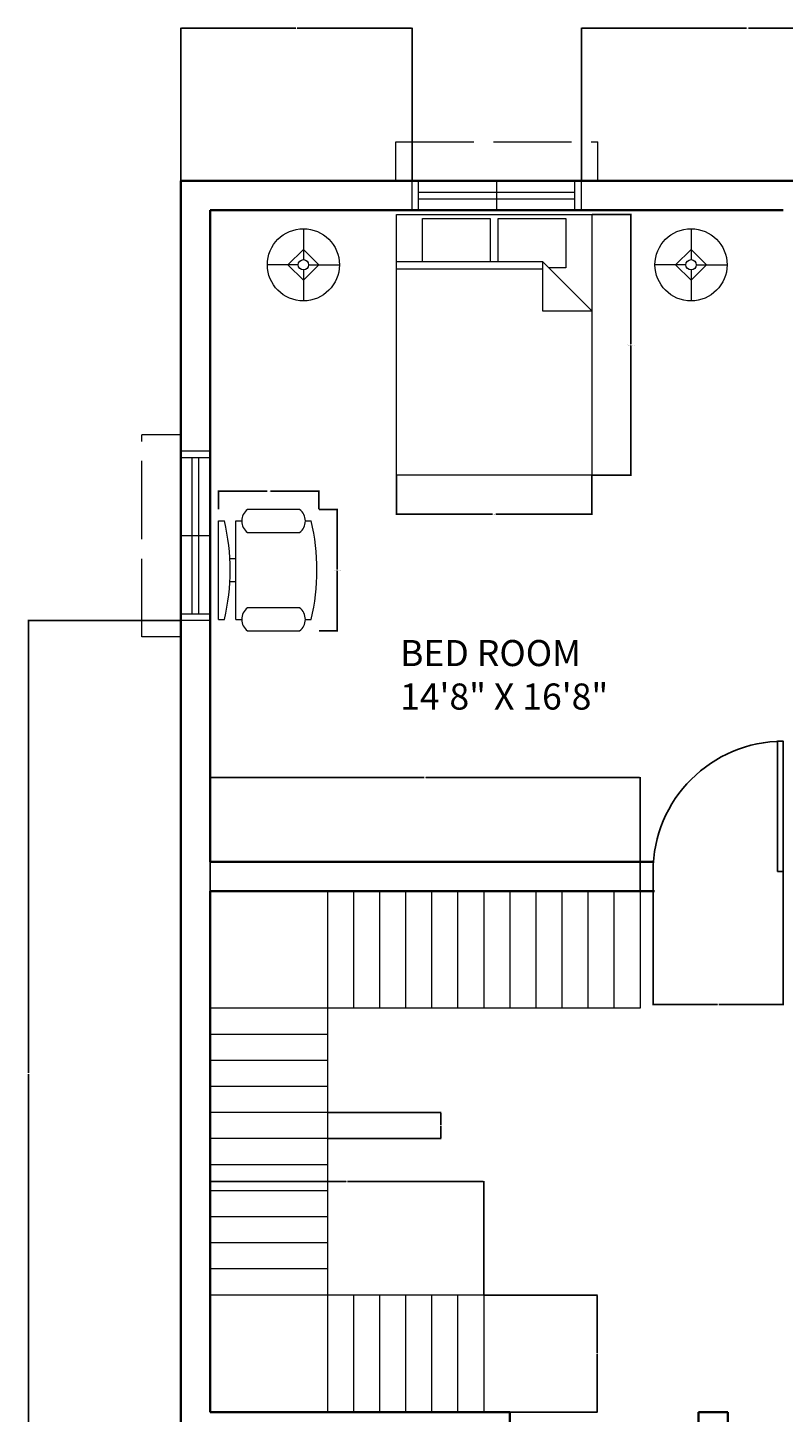
# Model space of a CAD drawing. Units: inches. Extents: x -1138 to 192, y 31 to 760.
# Tile 3 of 6: x -1138 to -906, y 323 to 748. Entities that reach past the tile are written whole.
import ezdxf

# ---------------------------------------------------------------- set-up
doc = ezdxf.new("R2010")
doc.units = ezdxf.units.IN
doc.header["$MEASUREMENT"] = 0
doc.linetypes.add('ACAD_ISO02W100', pattern=[15, 12, -3])
for name, color, linetype, lineweight in [('A-ANNO-DIMS', 2, 'Continuous', 18), ('A-AREA-IDEN', 7, 'Continuous', 18), ('A-DOOR', 3, 'Continuous', 25), ('A-FLOR-STRS', 7, 'Continuous', 18), ('A-FURN', 8, 'Continuous', 18), ('A-GLAZ', 4, 'Continuous', 20), ('A-GLAZ-OVHD', 4, 'ACAD_ISO02W100', 13), ('A-WALL', 7, 'Continuous', 35)]:
    doc.layers.add(name, color=color, linetype=linetype, lineweight=lineweight)
doc.styles.get("Standard").update_dxf_attribs({"font": 'arial.ttf'})
doc.dimstyles.get("Standard").update_dxf_attribs({"dimtxt": 0.18, "dimasz": 0.18, "dimexe": 0.18, "dimexo": 0.0625, "dimgap": 0.09, "dimtad": 0, "dimtih": 1, "dimtoh": 1, "dimdec": 1, "dimzin": 0, "dimdsep": 46, "dimlunit": 4, "dimtxsty": 'Standard', "dimcen": 0.09, "dimadec": 0, "dimazin": 0, "dimtfac": 1, "dimtdec": 1, "dimtofl": 0, "dimtmove": 0, "dimatfit": 3, "dimfxl": 1, "dimtolj": 1, "dimtzin": 0, "dimarcsym": 0})

# ---------------------------------------------------------------- blocks, each defined once
blk = doc.blocks.new('*U4')
for p, q in [((0, 0), (0, -6)), ((-40, 0), (-40, -6))]:
    blk.add_line(p, q)
blk.add_lwpolyline([(0, 0), (0, 40), (-1.75, 40), (-1.75, 0)], close=True)
blk.add_arc((0, 0), 40, 90, 180)
blk = doc.blocks.new('Bed - Queen')
for p, q in [((0, -80.00003), (0, 0)), ((0, 0), (59.99999, 0)), ((59.99999, 0), (59.99999, -80.00003)), ((7.99999, -1.2), (28.79998, -1.2)), ((7.99999, -14.4), (7.99999, -1.2)), ((28.79998, -1.2), (28.79998, -14.4)), ((31.19999, -1.2), (51.99999, -1.2)), ((31.19999, -14.4), (31.19999, -1.2)), ((51.99999, -1.2), (51.99999, -16.4)), ((0, -14.4), (44.8, -14.4)), ((44.8, -16.8), (0, -16.8)), ((59.99999, -29.6), (44.8, -14.4)), ((44.8, -14.4), (44.8, -29.6)), ((51.99999, -16.4), (46.79936, -16.4)), ((44.8, -29.6), (59.99999, -29.6)), ((59.99999, -80.00003), (0, -80.00003))]:
    blk.add_line(p, q)
blk = doc.blocks.new('Lamp - Table')
for p, q in [((0, 7), (0, 1)), ((0, 3), (-3, 0)), ((3, 0), (0, 3)), ((-1, 0), (-7, 0)), ((-3, 0), (0, -3)), ((0, -3), (3, 0)), ((1, 0), (7, 0)), ((0, -1), (0, -7))]:
    blk.add_line(p, q)
for radius in [7, 1]:
    blk.add_circle((0, 0), radius)
blk = doc.blocks.new('Chair - Desk')
for p, q in [((-8.5, 0), (-8.5, -1)), ((-8.5, 0), (8.5, 0)), ((8.5, 0), (8.5, -1)), ((-2, -3), (-2, -1.9355)), ((2, -1.9576), (2, -3)), ((-8.5, -3), (-8.5, -4)), ((-8.5, -3), (8.5, -3)), ((8.5, -3), (8.5, -4)), ((-10.5, -5), (-10.5, -14)), ((-6.5, -14), (-6.5, -5)), ((6.5, -5), (6.5, -14)), ((10.5, -14), (10.5, -5)), ((-8.5, -15), (-8.5, -16)), ((8.5, -15), (8.5, -16))]:
    blk.add_line(p, q)
for centre, radius, start, end in [((0, 34.625), 36.625, 256.5803, 283.4197), ((-8.5, -6.5), 2.5, 36.8699, 143.1301), ((8.5, -6.5), 2.5, 36.8699, 143.1301), ((-8.5, -12.5), 2.5, 216.8699, 323.1301), ((8.5, -12.5), 2.5, 216.8699, 323.1301), ((0, 19.625), 36.625, 256.5803, 283.4197)]:
    blk.add_arc(centre, radius, start, end)
blk = doc.blocks.new('WINDOW-48IN')
for p, q in [((0, 0), (0, 9)), ((2, 0), (2, 9)), ((26, 0), (26, 9)), ((50, 0), (50, 9)), ((52, 0), (52, 9)), ((2, 5.5), (50, 5.5)), ((2, 3.5), (50, 3.5))]:
    blk.add_line(p, q)
blk = doc.blocks.new('WINDOW-PROJECTION-62IN')
at = {"ltscale": 2}
for p, q in [((0, 0), (0, 12)), ((0, 12), (62, 12)), ((62, 0), (62, 12)), ((5, 0), (0, 0)), ((57, 0), (62, 0))]:
    blk.add_line(p, q, dxfattribs=at)
blk = doc.blocks.new('*D57')
at = {"layer": 'A-ANNO-DIMS', "color": 0, "lineweight": -2, "transparency": 16777216}
for p, q in [((-964.85, 690.45), (-952.73, 690.45)), ((-952.91, 690.27), (-952.91, 650.64)), ((-952.91, 610.63), (-952.91, 650.26)), ((-964.85, 610.45), (-952.73, 610.45))]:
    blk.add_line(p, q, dxfattribs=at)
at = {"layer": 'A-ANNO-DIMS', "color": 0, "transparency": 16777216}
for points in [[(-952.94, 690.27), (-952.88, 690.27), (-952.91, 690.45)], [(-952.94, 610.63), (-952.88, 610.63), (-952.91, 610.45)]]:
    blk.add_solid(points, dxfattribs=at)
at = {"layer": 'Defpoints', "color": 0, "transparency": 16777216}
for p in [(-964.91, 690.45), (-952.91, 690.45), (-964.91, 610.45)]:
    blk.add_point(p, dxfattribs=at)
at = {"layer": 'A-ANNO-DIMS', "color": 0, "transparency": 16777216, "insert": (-952.91, 650.45), "char_height": 0.18, "attachment_point": 5}
blk.add_mtext('\\A1;QUEEN BED 80 TYP.', dxfattribs=at)
blk = doc.blocks.new('*D58')
at = {"layer": 'A-ANNO-DIMS', "color": 0, "lineweight": -2, "transparency": 16777216}
for p, q in [((-1024.91, 610.39), (-1024.91, 598.27)), ((-964.91, 610.39), (-964.91, 598.27)), ((-1024.73, 598.45), (-995.44, 598.45)), ((-965.09, 598.45), (-994.38, 598.45))]:
    blk.add_line(p, q, dxfattribs=at)
at = {"layer": 'A-ANNO-DIMS', "color": 0, "transparency": 16777216}
for points in [[(-1024.73, 598.48), (-1024.73, 598.42), (-1024.91, 598.45)], [(-965.09, 598.48), (-965.09, 598.42), (-964.91, 598.45)]]:
    blk.add_solid(points, dxfattribs=at)
at = {"layer": 'Defpoints', "color": 0, "transparency": 16777216}
for p in [(-1024.91, 610.45), (-964.91, 610.45), (-964.91, 598.45)]:
    blk.add_point(p, dxfattribs=at)
at = {"layer": 'A-ANNO-DIMS', "color": 0, "transparency": 16777216, "insert": (-994.91, 598.45), "char_height": 0.18, "attachment_point": 5}
blk.add_mtext('\\A1;60 TYP.', dxfattribs=at)
blk = doc.blocks.new('*D59')
at = {"layer": 'A-ANNO-DIMS', "color": 0, "lineweight": -2, "transparency": 16777216}
for p, q in [((-1048.67, 599.95), (-1042.96, 599.95)), ((-1043.14, 599.77), (-1043.14, 581.47)), ((-1043.14, 562.81), (-1043.14, 581.11)), ((-1048.67, 562.63), (-1042.96, 562.63))]:
    blk.add_line(p, q, dxfattribs=at)
at = {"layer": 'A-ANNO-DIMS', "color": 0, "transparency": 16777216}
for points in [[(-1043.17, 599.77), (-1043.11, 599.77), (-1043.14, 599.95)], [(-1043.17, 562.81), (-1043.11, 562.81), (-1043.14, 562.63)]]:
    blk.add_solid(points, dxfattribs=at)
at = {"layer": 'Defpoints', "color": 0, "transparency": 16777216}
for p in [(-1048.74, 599.95), (-1043.14, 599.95), (-1048.74, 562.63)]:
    blk.add_point(p, dxfattribs=at)
at = {"layer": 'A-ANNO-DIMS', "color": 0, "transparency": 16777216, "insert": (-1043.14, 581.29), "char_height": 0.18, "attachment_point": 5}
blk.add_mtext('\\A1;DESK CHAIR 37 TYP.', dxfattribs=at)
blk = doc.blocks.new('*D60')
at = {"layer": 'A-ANNO-DIMS', "color": 0, "lineweight": -2, "transparency": 16777216}
for p, q in [((-1079.53, 600.01), (-1079.53, 605.72)), ((-1079.35, 605.54), (-1064.66, 605.54)), ((-1048.92, 605.54), (-1063.61, 605.54)), ((-1048.74, 600.01), (-1048.74, 605.72))]:
    blk.add_line(p, q, dxfattribs=at)
at = {"layer": 'A-ANNO-DIMS', "color": 0, "transparency": 16777216}
for points in [[(-1079.35, 605.57), (-1079.35, 605.51), (-1079.53, 605.54)], [(-1048.92, 605.57), (-1048.92, 605.51), (-1048.74, 605.54)]]:
    blk.add_solid(points, dxfattribs=at)
at = {"layer": 'Defpoints', "color": 0, "transparency": 16777216}
for p in [(-1079.53, 605.54), (-1079.53, 599.95), (-1048.74, 599.95)]:
    blk.add_point(p, dxfattribs=at)
at = {"layer": 'A-ANNO-DIMS', "color": 0, "transparency": 16777216, "insert": (-1064.13, 605.54), "char_height": 0.18, "attachment_point": 5}
blk.add_mtext('\\A1;31 TYP.', dxfattribs=at)
blk = doc.blocks.new('*D87')
at = {"layer": 'A-ANNO-DIMS', "color": 0, "lineweight": -2, "transparency": 16777216}
for p, q in [((-1091.13, 700.88), (-1091.13, 747.81)), ((-1090.95, 747.63), (-1055.83, 747.63)), ((-1020.31, 747.63), (-1055.43, 747.63)), ((-1020.13, 700.88), (-1020.13, 747.81))]:
    blk.add_line(p, q, dxfattribs=at)
at = {"layer": 'A-ANNO-DIMS', "color": 0, "transparency": 16777216}
for points in [[(-1090.95, 747.66), (-1090.95, 747.6), (-1091.13, 747.63)], [(-1020.31, 747.66), (-1020.31, 747.6), (-1020.13, 747.63)]]:
    blk.add_solid(points, dxfattribs=at)
at = {"layer": 'Defpoints', "color": 0, "transparency": 16777216}
for p in [(-1020.13, 747.63), (-1091.13, 700.81), (-1020.13, 700.81)]:
    blk.add_point(p, dxfattribs=at)
at = {"layer": 'A-ANNO-DIMS', "color": 0, "transparency": 16777216, "insert": (-1055.63, 747.63), "char_height": 0.18, "attachment_point": 5}
blk.add_mtext('\\A1;71', dxfattribs=at)
blk = doc.blocks.new('*D88')
at = {"layer": 'A-ANNO-DIMS', "color": 0, "lineweight": -2, "transparency": 16777216}
for p, q in [((-968.13, 700.88), (-968.13, 747.81)), ((-967.95, 747.63), (-917.41, 747.63)), ((-866.31, 747.63), (-916.85, 747.63)), ((-866.13, 700.88), (-866.13, 747.81))]:
    blk.add_line(p, q, dxfattribs=at)
at = {"layer": 'A-ANNO-DIMS', "color": 0, "transparency": 16777216}
for points in [[(-967.95, 747.66), (-967.95, 747.6), (-968.13, 747.63)], [(-866.31, 747.66), (-866.31, 747.6), (-866.13, 747.63)]]:
    blk.add_solid(points, dxfattribs=at)
at = {"layer": 'Defpoints', "color": 0, "transparency": 16777216}
for p in [(-866.13, 747.63), (-968.13, 700.81), (-866.13, 700.81)]:
    blk.add_point(p, dxfattribs=at)
at = {"layer": 'A-ANNO-DIMS', "color": 0, "transparency": 16777216, "insert": (-917.13, 747.63), "char_height": 0.18, "attachment_point": 5}
blk.add_mtext('\\A1;102', dxfattribs=at)
blk = doc.blocks.new('*D94')
at = {"layer": 'A-ANNO-DIMS', "color": 0, "lineweight": -2, "transparency": 16777216}
for p, q in [((-1091.2, 565.81), (-1138.13, 565.81)), ((-1137.95, 565.63), (-1137.95, 426.99)), ((-1137.95, 287.99), (-1137.95, 426.63)), ((-1091.2, 287.81), (-1138.13, 287.81))]:
    blk.add_line(p, q, dxfattribs=at)
at = {"layer": 'A-ANNO-DIMS', "color": 0, "transparency": 16777216}
for points in [[(-1137.98, 565.63), (-1137.92, 565.63), (-1137.95, 565.81)], [(-1137.98, 287.99), (-1137.92, 287.99), (-1137.95, 287.81)]]:
    blk.add_solid(points, dxfattribs=at)
at = {"layer": 'Defpoints', "color": 0, "transparency": 16777216}
for p in [(-1137.95, 565.81), (-1091.13, 565.81), (-1091.13, 287.81)]:
    blk.add_point(p, dxfattribs=at)
at = {"layer": 'A-ANNO-DIMS', "color": 0, "transparency": 16777216, "insert": (-1137.95, 426.81), "char_height": 0.18, "attachment_point": 5}
blk.add_mtext('\\A1;278', dxfattribs=at)
blk = doc.blocks.new('*D99')
at = {"layer": 'A-ANNO-DIMS', "color": 0, "lineweight": -2, "transparency": 16777216}
for p, q in [((-946.13, 482.75), (-946.13, 447.82)), ((-906.13, 482.75), (-906.13, 447.82)), ((-945.95, 448), (-926.36, 448)), ((-906.31, 448), (-925.91, 448))]:
    blk.add_line(p, q, dxfattribs=at)
at = {"layer": 'A-ANNO-DIMS', "color": 0, "transparency": 16777216}
for points in [[(-945.95, 448.03), (-945.95, 447.97), (-946.13, 448)], [(-906.31, 448.03), (-906.31, 447.97), (-906.13, 448)]]:
    blk.add_solid(points, dxfattribs=at)
at = {"layer": 'Defpoints', "color": 0, "transparency": 16777216}
for p in [(-946.13, 482.81), (-906.13, 482.81), (-946.13, 448)]:
    blk.add_point(p, dxfattribs=at)
at = {"layer": 'A-ANNO-DIMS', "color": 0, "transparency": 16777216, "insert": (-926.13, 448), "char_height": 0.18, "attachment_point": 5}
blk.add_mtext('\\A1;40', dxfattribs=at)
blk = doc.blocks.new('*D101')
at = {"layer": 'A-ANNO-DIMS', "color": 0, "lineweight": -2, "transparency": 16777216}
for p, q in [((-998.07, 358.81), (-963.14, 358.81)), ((-963.32, 358.63), (-963.32, 340.99)), ((-963.32, 322.99), (-963.32, 340.63)), ((-998.07, 322.81), (-963.14, 322.81))]:
    blk.add_line(p, q, dxfattribs=at)
at = {"layer": 'A-ANNO-DIMS', "color": 0, "transparency": 16777216}
for points in [[(-963.35, 358.63), (-963.29, 358.63), (-963.32, 358.81)], [(-963.35, 322.99), (-963.29, 322.99), (-963.32, 322.81)]]:
    blk.add_solid(points, dxfattribs=at)
at = {"layer": 'Defpoints', "color": 0, "transparency": 16777216}
for p in [(-998.13, 358.81), (-998.13, 322.81), (-963.32, 322.81)]:
    blk.add_point(p, dxfattribs=at)
at = {"layer": 'A-ANNO-DIMS', "color": 0, "transparency": 16777216, "insert": (-963.32, 340.81), "char_height": 0.18, "attachment_point": 5}
blk.add_mtext('\\A1;36', dxfattribs=at)
blk = doc.blocks.new('*D102')
at = {"layer": 'A-ANNO-DIMS', "color": 0, "lineweight": -2, "transparency": 16777216}
for p, q in [((-1082.13, 482.88), (-1082.13, 517.81)), ((-1081.95, 517.63), (-1016.41, 517.63)), ((-950.31, 517.63), (-1015.85, 517.63)), ((-950.13, 482.88), (-950.13, 517.81))]:
    blk.add_line(p, q, dxfattribs=at)
at = {"layer": 'A-ANNO-DIMS', "color": 0, "transparency": 16777216}
for points in [[(-1081.95, 517.66), (-1081.95, 517.6), (-1082.13, 517.63)], [(-950.31, 517.66), (-950.31, 517.6), (-950.13, 517.63)]]:
    blk.add_solid(points, dxfattribs=at)
at = {"layer": 'Defpoints', "color": 0, "transparency": 16777216}
for p in [(-950.13, 517.63), (-1082.13, 482.81), (-950.13, 482.81)]:
    blk.add_point(p, dxfattribs=at)
at = {"layer": 'A-ANNO-DIMS', "color": 0, "transparency": 16777216, "insert": (-1016.13, 517.63), "char_height": 0.18, "attachment_point": 5}
blk.add_mtext('\\A1;132', dxfattribs=at)
blk = doc.blocks.new('*D103')
at = {"layer": 'A-ANNO-DIMS', "color": 0, "lineweight": -2, "transparency": 16777216}
for p, q in [((-1046.07, 414.81), (-1011.14, 414.81)), ((-1011.32, 414.63), (-1011.32, 410.99)), ((-1011.32, 406.99), (-1011.32, 410.63)), ((-1046.07, 406.81), (-1011.14, 406.81))]:
    blk.add_line(p, q, dxfattribs=at)
at = {"layer": 'A-ANNO-DIMS', "color": 0, "transparency": 16777216}
for points in [[(-1011.35, 414.63), (-1011.29, 414.63), (-1011.32, 414.81)], [(-1011.35, 406.99), (-1011.29, 406.99), (-1011.32, 406.81)]]:
    blk.add_solid(points, dxfattribs=at)
at = {"layer": 'Defpoints', "color": 0, "transparency": 16777216}
for p in [(-1046.13, 414.81), (-1046.13, 406.81), (-1011.32, 406.81)]:
    blk.add_point(p, dxfattribs=at)
at = {"layer": 'A-ANNO-DIMS', "color": 0, "transparency": 16777216, "insert": (-1011.32, 410.81), "char_height": 0.18, "attachment_point": 5}
blk.add_mtext('\\A1;8', dxfattribs=at)
blk = doc.blocks.new('*D104')
at = {"layer": 'A-ANNO-DIMS', "color": 0, "lineweight": -2, "transparency": 16777216}
for p, q in [((-1082.13, 358.88), (-1082.13, 393.81)), ((-1081.95, 393.63), (-1040.35, 393.63)), ((-998.31, 393.63), (-1039.91, 393.63)), ((-998.13, 358.88), (-998.13, 393.81))]:
    blk.add_line(p, q, dxfattribs=at)
at = {"layer": 'A-ANNO-DIMS', "color": 0, "transparency": 16777216}
for points in [[(-1081.95, 393.66), (-1081.95, 393.6), (-1082.13, 393.63)], [(-998.31, 393.66), (-998.31, 393.6), (-998.13, 393.63)]]:
    blk.add_solid(points, dxfattribs=at)
at = {"layer": 'Defpoints', "color": 0, "transparency": 16777216}
for p in [(-998.13, 393.63), (-1082.13, 358.81), (-998.13, 358.81)]:
    blk.add_point(p, dxfattribs=at)
at = {"layer": 'A-ANNO-DIMS', "color": 0, "transparency": 16777216, "insert": (-1040.13, 393.63), "char_height": 0.18, "attachment_point": 5}
blk.add_mtext('\\A1;84', dxfattribs=at)

msp = doc.modelspace()

# ---------------------------------------------------------------- linework, layer by layer
at = {"layer": 'A-FLOR-STRS'}
for p, q in [((-1046.133, 482.813), (-1046.133, 322.813)), ((-1038.133, 482.813), (-1038.133, 446.813)), ((-1030.133, 482.813), (-1030.133, 446.813)), ((-1022.133, 482.813), (-1022.133, 446.813)), ((-1014.133, 482.813), (-1014.133, 446.813)), ((-1006.133, 482.813), (-1006.133, 446.813)), ((-998.133, 482.813), (-998.133, 446.813)), ((-990.133, 482.813), (-990.133, 446.813)), ((-982.133, 482.813), (-982.133, 446.813)), ((-974.133, 482.813), (-974.133, 446.813)), ((-966.133, 482.813), (-966.133, 446.813)), ((-958.133, 482.813), (-958.133, 446.813)), ((-950.133, 482.813), (-950.133, 446.813)), ((-950.133, 446.813), (-1082.133, 446.813)), ((-1046.133, 438.813), (-1082.133, 438.813)), ((-1046.133, 430.813), (-1082.133, 430.813)), ((-1046.133, 422.813), (-1082.133, 422.813)), ((-1046.133, 414.813), (-1082.133, 414.813)), ((-1046.133, 406.813), (-1082.133, 406.813)), ((-1046.133, 398.813), (-1082.133, 398.813)), ((-1046.133, 390.813), (-1082.133, 390.813)), ((-1046.133, 382.813), (-1082.133, 382.813)), ((-1046.133, 374.813), (-1082.133, 374.813)), ((-1046.133, 366.813), (-1082.133, 366.813)), ((-998.133, 358.813), (-1082.133, 358.813)), ((-1038.133, 358.813), (-1038.133, 322.813)), ((-1030.133, 358.813), (-1030.133, 322.813)), ((-1022.133, 358.813), (-1022.133, 322.813)), ((-1014.133, 358.813), (-1014.133, 322.813)), ((-1006.133, 358.813), (-1006.133, 322.813)), ((-998.133, 358.813), (-998.133, 322.813))]:
    msp.add_line(p, q, dxfattribs=at)
at = {"layer": 'A-WALL'}
for p, q in [((-1091.133, 700.813), (-897.133, 700.813)), ((-1091.133, 491.813), (-1091.133, 700.813)), ((-1082.133, 691.813), (-906.133, 691.813)), ((-1082.133, 491.813), (-1082.133, 691.813)), ((-1091.133, 491.813), (-1091.133, 294.813)), ((-946.02, 491.813), (-1082.133, 491.813)), ((-946.02, 491.813), (-1082.133, 491.813)), ((-1082.133, 482.813), (-1082.133, 322.813)), ((-945.68, 482.813), (-1082.133, 482.813)), ((-990.133, 322.813), (-1082.133, 322.813)), ((-990.133, 224.813), (-990.133, 322.813)), ((-932.133, 86.813), (-932.133, 322.813)), ((-923.133, 322.813), (-932.133, 322.813)), ((-923.133, 313.813), (-923.133, 322.813))]:
    msp.add_line(p, q, dxfattribs=at)

# ---------------------------------------------------------------- block references
at = {"layer": 'A-DOOR'}
msp.add_blockref('*U4', (-906.133, 488.813), dxfattribs=at)
at = {"layer": 'A-FURN'}
msp.add_blockref('Bed - Queen', (-1024.911, 690.45), dxfattribs=at)
at = {"layer": 'A-FURN', "xscale": 1.581140411223051, "yscale": 1.581140411223051, "zscale": 1.581140411223051}
for p in [(-1053.494, 675.031), (-934.47, 675.031)]:
    msp.add_blockref('Lamp - Table', p, dxfattribs=at)
at = {"layer": 'A-FURN', "xscale": 1.776798148379839, "yscale": 1.776798148379839, "zscale": 1.776798148379839, "rotation": 90}
msp.add_blockref('Chair - Desk', (-1079.533, 581.291), dxfattribs=at)
at = {"layer": 'A-GLAZ'}
msp.add_blockref('WINDOW-48IN', (-1020.133, 691.813), dxfattribs=at)
at = {"layer": 'A-GLAZ', "rotation": 89.9999999999989}
msp.add_blockref('WINDOW-48IN', (-1082.133, 565.813), dxfattribs=at)
at = {"layer": 'A-GLAZ-OVHD'}
msp.add_blockref('WINDOW-PROJECTION-62IN', (-1025.133, 700.813), dxfattribs=at)
at = {"layer": 'A-GLAZ-OVHD', "rotation": 89.99999999999925}
msp.add_blockref('WINDOW-PROJECTION-62IN', (-1091.133, 560.813), dxfattribs=at)

# ---------------------------------------------------------------- texts
at = {"layer": 'A-AREA-IDEN', "insert": (-1023.799, 559.856), "char_height": 8, "attachment_point": 1}
msp.add_mtext_dynamic_manual_height_columns('BED ROOM\\P14\'8" X 16\'8"', width=126.58932, gutter_width=1, heights=[0], dxfattribs=at)

# ---------------------------------------------------------------- dimensions: what is measured, and where the dimension line sits
at = {"layer": 'A-ANNO-DIMS'}
for base, p1, p2, picture, middle in [((-1020.133, 747.628), (-1091.133, 700.813), (-1020.133, 700.813), '*D87', (-1055.633, 747.628)), ((-866.133, 747.628), (-968.133, 700.813), (-866.133, 700.813), '*D88', (-917.133, 747.628)), ((-950.133, 517.628), (-1082.133, 482.813), (-950.133, 482.813), '*D102', (-1016.133, 517.628)), ((-998.133, 393.628), (-1082.133, 358.813), (-998.133, 358.813), '*D104', (-1040.133, 393.628))]:
    dim = msp.add_linear_dim(base=base, p1=p1, p2=p2, dimstyle='Standard', override={"dimdec": 0, "dimlfac": 1, "dimrnd": 0, "dimzin": 0, "dimdsep": 46, "dimlunit": 2}, dxfattribs=at)
    dim.commit()
    dim.dimension.update_dxf_attribs({"geometry": picture, "text_midpoint": middle})
for base, p1, p2, angle, text, picture, middle in [((-952.911, 690.45), (-964.911, 610.45), (-964.911, 690.45), 90, 'QUEEN BED <> TYP.', '*D57', (-952.911, 650.45)), ((-1079.533, 605.544), (-1048.735, 599.947), (-1079.533, 599.947), 180, '<> TYP.', '*D60', (-1064.134, 605.544)), ((-1043.139, 599.947), (-1048.735, 562.635), (-1048.735, 599.947), 90, 'DESK CHAIR <> TYP.', '*D59', (-1043.139, 581.291))]:
    dim = msp.add_linear_dim(base=base, p1=p1, p2=p2, angle=angle, text=text, dimstyle='Standard', override={"dimdec": 0, "dimlfac": 1, "dimrnd": 0, "dimzin": 0, "dimdsep": 46, "dimlunit": 2}, dxfattribs=at)
    dim.commit()
    dim.dimension.update_dxf_attribs({"geometry": picture, "text_midpoint": middle})
dim = msp.add_linear_dim(base=(-964.911, 598.45), p1=(-1024.911, 610.45), p2=(-964.911, 610.45), text='<> TYP.', dimstyle='Standard', override={"dimdec": 0, "dimlfac": 1, "dimrnd": 0, "dimzin": 0, "dimdsep": 46, "dimlunit": 2}, dxfattribs=at)
dim.commit()
dim.dimension.update_dxf_attribs({"geometry": '*D58', "text_midpoint": (-994.911, 598.45)})
for base, p1, p2, angle, picture, middle in [((-1137.948, 565.813), (-1091.133, 287.813), (-1091.133, 565.813), 90, '*D94', (-1137.948, 426.813)), ((-946.133, 447.998), (-906.133, 482.813), (-946.133, 482.813), 180, '*D99', (-926.133, 447.998)), ((-1011.318, 406.813), (-1046.133, 414.813), (-1046.133, 406.813), 270, '*D103', (-1011.318, 410.813)), ((-963.318, 322.813), (-998.133, 358.813), (-998.133, 322.813), 270, '*D101', (-963.318, 340.813))]:
    dim = msp.add_linear_dim(base=base, p1=p1, p2=p2, angle=angle, dimstyle='Standard', override={"dimdec": 0, "dimlfac": 1, "dimrnd": 0, "dimzin": 0, "dimdsep": 46, "dimlunit": 2}, dxfattribs=at)
    dim.commit()
    dim.dimension.update_dxf_attribs({"geometry": picture, "text_midpoint": middle})

doc.saveas('drawing.dxf')
